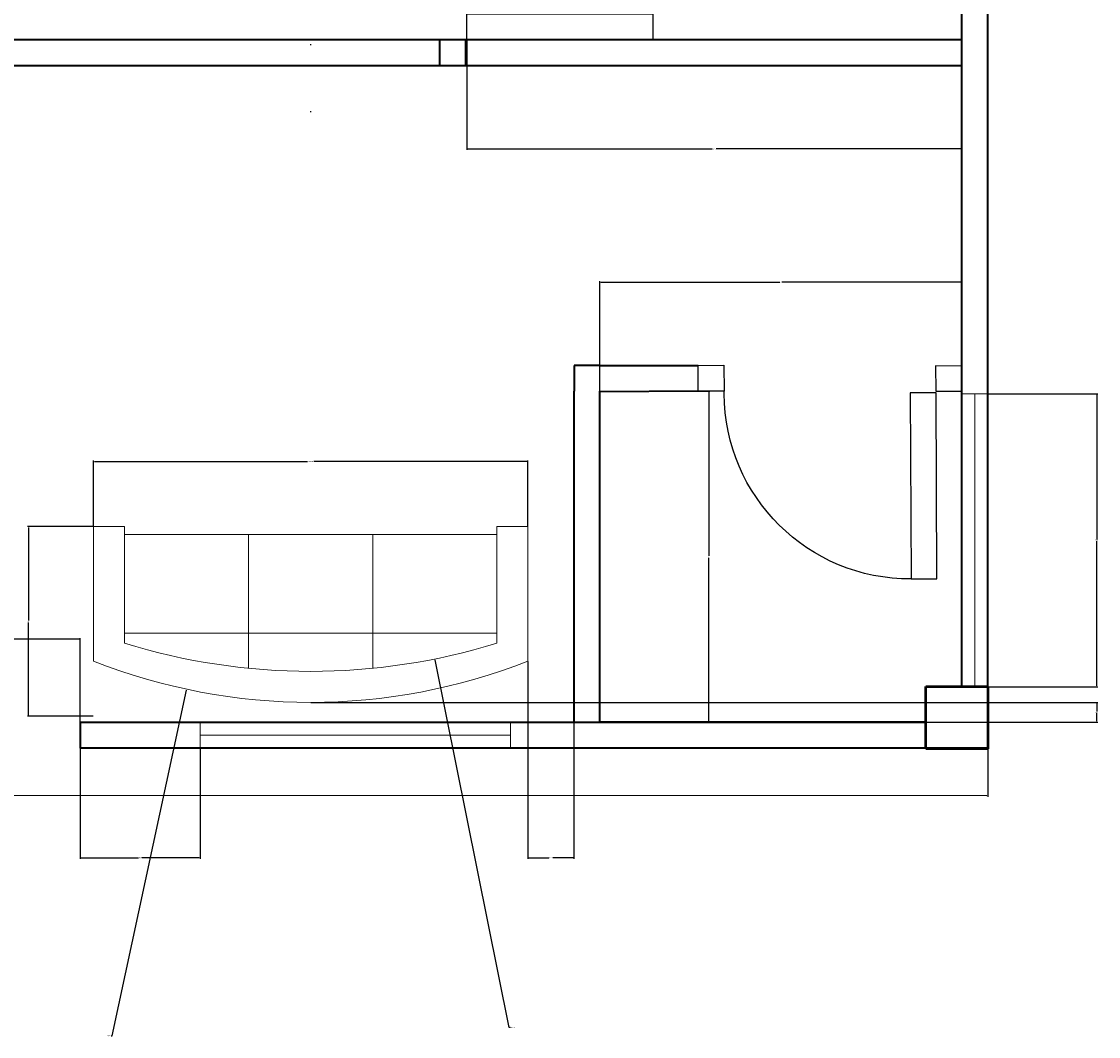
# Model space of a CAD drawing. Units: inches. Extents: x 2082 to 2506, y 790 to 1201.
# Tile 2 of 3: x 2298 to 2506, y 790 to 986. Entities that reach past the tile are written whole.
import ezdxf

# ---------------------------------------------------------------- set-up
doc = ezdxf.new("R2010")
doc.units = ezdxf.units.IN
for name, color, linetype, lineweight in [('A-ANNO-DIMS', 2, 'Continuous', 18), ('A-COLS', 7, 'Continuous', 50), ('A-DOOR', 3, 'Continuous', 25), ('A-FURN', 8, 'Continuous', 18), ('A-GLAZ', 4, 'Continuous', 18), ('A-WALL', 7, 'Continuous', 35)]:
    doc.layers.add(name, color=color, linetype=linetype, lineweight=lineweight)
doc.styles.get("Standard").update_dxf_attribs({"font": 'arial.ttf'})
doc.dimstyles.get("Standard").update_dxf_attribs({"dimtxt": 0.18, "dimasz": 0.18, "dimexe": 0.18, "dimexo": 0.0625, "dimgap": 0.09, "dimtad": 0, "dimtih": 1, "dimtoh": 1, "dimdec": 4, "dimzin": 0, "dimdsep": 46, "dimlunit": 4, "dimtxsty": 'Standard', "dimcen": 0.09, "dimadec": 0, "dimazin": 0, "dimtfac": 1, "dimtdec": 4, "dimtofl": 0, "dimtmove": 0, "dimatfit": 3, "dimfxl": 1, "dimtolj": 1, "dimtzin": 0, "dimarcsym": 0})

# ---------------------------------------------------------------- blocks, each defined once
blk = doc.blocks.new('Sofa - Roundback 7 ft.')
for p, q in [((-12.00002, -32.4421), (-12.00003, -6.5971)), ((11.99997, -32.4421), (11.99998, -6.5971)), ((-36.000027, -34), (-36.000027, -11.4696)), ((35.99998, -34), (35.99998, -11.4696)), ((-35.999844, -13.3819), (35.9998, -13.3819)), ((-36.000027, -32.4421), (35.99998, -32.4421))]:
    blk.add_line(p, q)
for points in [[(-36.000027, -34), (-42.000027, -34), (-42.000027, -8)], [(41.99998, -8), (41.99998, -34), (35.99998, -34)]]:
    blk.add_lwpolyline(points)
for centre, radius, start, end in [((0, -114.25), 114.25, 68.43141, 111.5686), ((-0.00001, -127.1968), 121.1968, 72.72033, 107.2797)]:
    blk.add_arc(centre, radius, start, end)
blk = doc.blocks.new('DOOR-SWING-36IN')
for p, q in [((0, 0), (0, 5)), ((0, 5), (36, 5)), ((36, 5), (36, 0)), ((36, 0), (0, 0))]:
    blk.add_line(p, q)
blk.add_arc((0, 5), 36, 0, 90)
blk = doc.blocks.new('WIN-60IN')
for p, q in [((0, 5), (12, 5)), ((0, 5), (0, 0)), ((12, 5), (60, 5)), ((60, 5), (60, 0)), ((0, 2.5), (60, 2.5)), ((0, 0), (60, 0))]:
    blk.add_line(p, q)
blk = doc.blocks.new('COL-12X12IN')
for p, q in [((0, 12), (12, 12)), ((0, 0), (0, 12)), ((12, 12), (12, 0)), ((12, 0), (0, 0))]:
    blk.add_line(p, q)
blk = doc.blocks.new('*D22')
at = {"layer": 'A-ANNO-DIMS', "color": 0, "lineweight": -2, "transparency": 16777216}
for p, q in [((2311.99, 888.4), (2311.99, 901.12)), ((2312.17, 900.94), (2353.4, 900.94)), ((2395.81, 900.94), (2354.59, 900.94)), ((2395.99, 888.4), (2395.99, 901.12))]:
    blk.add_line(p, q, dxfattribs=at)
at = {"layer": 'A-ANNO-DIMS', "color": 0, "transparency": 16777216}
for points in [[(2312.17, 900.97), (2312.17, 900.91), (2311.99, 900.94)], [(2395.81, 900.97), (2395.81, 900.91), (2395.99, 900.94)]]:
    blk.add_solid(points, dxfattribs=at)
at = {"layer": 'Defpoints', "color": 0, "transparency": 16777216}
for p in [(2311.99, 900.94), (2311.99, 888.34), (2395.99, 888.34)]:
    blk.add_point(p, dxfattribs=at)
at = {"layer": 'A-ANNO-DIMS', "color": 0, "transparency": 16777216, "insert": (2353.99, 900.94), "char_height": 0.18, "attachment_point": 5}
blk.add_mtext('\\A1;SOFA 84', dxfattribs=at)
blk = doc.blocks.new('*D23')
at = {"layer": 'A-ANNO-DIMS', "color": 0, "lineweight": -2, "transparency": 16777216}
for p, q in [((2311.93, 888.34), (2299.21, 888.34)), ((2299.39, 888.16), (2299.39, 870.19)), ((2299.39, 851.85), (2299.39, 869.82)), ((2311.93, 851.67), (2299.21, 851.67))]:
    blk.add_line(p, q, dxfattribs=at)
at = {"layer": 'A-ANNO-DIMS', "color": 0, "transparency": 16777216}
for points in [[(2299.36, 888.16), (2299.42, 888.16), (2299.39, 888.34)], [(2299.36, 851.85), (2299.42, 851.85), (2299.39, 851.67)]]:
    blk.add_solid(points, dxfattribs=at)
at = {"layer": 'Defpoints', "color": 0, "transparency": 16777216}
for p in [(2311.99, 888.34), (2299.39, 851.67), (2311.99, 851.67)]:
    blk.add_point(p, dxfattribs=at)
at = {"layer": 'A-ANNO-DIMS', "color": 0, "transparency": 16777216, "insert": (2299.39, 870), "char_height": 0.18, "attachment_point": 5}
blk.add_mtext('\\A1;37', dxfattribs=at)
blk = doc.blocks.new('*D24')
at = {"layer": 'A-ANNO-DIMS', "color": 0, "lineweight": -2, "transparency": 16777216}
for p, q in [((2102.92, 857.43), (2102.92, 836.21)), ((2484.95, 857.32), (2484.95, 836.1)), ((2103.1, 836.39), (2293.64, 836.34)), ((2484.77, 836.28), (2294.22, 836.34))]:
    blk.add_line(p, q, dxfattribs=at)
at = {"layer": 'A-ANNO-DIMS', "color": 0, "transparency": 16777216}
for points in [[(2103.1, 836.42), (2103.1, 836.36), (2102.92, 836.39)], [(2484.77, 836.31), (2484.77, 836.25), (2484.95, 836.28)]]:
    blk.add_solid(points, dxfattribs=at)
at = {"layer": 'Defpoints', "color": 0, "transparency": 16777216}
for p in [(2102.92, 857.49), (2484.95, 857.38), (2102.92, 836.39)]:
    blk.add_point(p, dxfattribs=at)
at = {"layer": 'A-ANNO-DIMS', "color": 0, "transparency": 16777216, "insert": (2293.93, 836.34), "char_height": 0.18, "attachment_point": 5}
blk.add_mtext('\\A1;382', dxfattribs=at)
blk = doc.blocks.new('*D36')
at = {"layer": 'A-ANNO-DIMS', "color": 0, "lineweight": -2, "transparency": 16777216}
for p, q in [((2384.17, 982.44), (2384.17, 961.22)), ((2479.92, 982.44), (2479.92, 961.22)), ((2384.35, 961.4), (2431.65, 961.4)), ((2479.74, 961.4), (2432.44, 961.4))]:
    blk.add_line(p, q, dxfattribs=at)
at = {"layer": 'A-ANNO-DIMS', "color": 0, "transparency": 16777216}
for points in [[(2384.35, 961.43), (2384.35, 961.37), (2384.17, 961.4)], [(2479.74, 961.43), (2479.74, 961.37), (2479.92, 961.4)]]:
    blk.add_solid(points, dxfattribs=at)
at = {"layer": 'Defpoints', "color": 0, "transparency": 16777216}
for p in [(2384.17, 982.5), (2479.92, 982.5), (2384.17, 961.4)]:
    blk.add_point(p, dxfattribs=at)
at = {"layer": 'A-ANNO-DIMS', "color": 0, "transparency": 16777216, "insert": (2432.05, 961.4), "char_height": 0.18, "attachment_point": 5}
blk.add_mtext('\\A1;95.75', dxfattribs=at)
blk = doc.blocks.new('*D37')
at = {"layer": 'A-ANNO-DIMS', "color": 0, "lineweight": -2, "transparency": 16777216}
for p, q in [((2409.92, 914.56), (2409.92, 935.78)), ((2410.1, 935.6), (2444.71, 935.6)), ((2479.74, 935.6), (2445.14, 935.6)), ((2479.92, 914.56), (2479.92, 935.78))]:
    blk.add_line(p, q, dxfattribs=at)
at = {"layer": 'A-ANNO-DIMS', "color": 0, "transparency": 16777216}
for points in [[(2410.1, 935.63), (2410.1, 935.57), (2409.92, 935.6)], [(2479.74, 935.63), (2479.74, 935.57), (2479.92, 935.6)]]:
    blk.add_solid(points, dxfattribs=at)
at = {"layer": 'Defpoints', "color": 0, "transparency": 16777216}
for p in [(2479.92, 935.6), (2409.92, 914.5), (2479.92, 914.5)]:
    blk.add_point(p, dxfattribs=at)
at = {"layer": 'A-ANNO-DIMS', "color": 0, "transparency": 16777216, "insert": (2444.92, 935.6), "char_height": 0.18, "attachment_point": 5}
blk.add_mtext('\\A1;70', dxfattribs=at)
blk = doc.blocks.new('*D38')
at = {"layer": 'A-ANNO-DIMS', "color": 0, "lineweight": -2, "transparency": 16777216}
for p, q in [((2409.99, 914.5), (2431.2, 914.5)), ((2431.02, 914.32), (2431.02, 882.68)), ((2431.02, 850.68), (2431.02, 882.32)), ((2409.99, 850.5), (2431.2, 850.5))]:
    blk.add_line(p, q, dxfattribs=at)
at = {"layer": 'A-ANNO-DIMS', "color": 0, "transparency": 16777216}
for points in [[(2430.99, 914.32), (2431.05, 914.32), (2431.02, 914.5)], [(2430.99, 850.68), (2431.05, 850.68), (2431.02, 850.5)]]:
    blk.add_solid(points, dxfattribs=at)
at = {"layer": 'Defpoints', "color": 0, "transparency": 16777216}
for p in [(2409.92, 914.5), (2409.92, 850.5), (2431.02, 850.5)]:
    blk.add_point(p, dxfattribs=at)
at = {"layer": 'A-ANNO-DIMS', "color": 0, "transparency": 16777216, "insert": (2431.02, 882.5), "char_height": 0.18, "attachment_point": 5}
blk.add_mtext('\\A1;64', dxfattribs=at)
blk = doc.blocks.new('*D41')
at = {"layer": 'A-ANNO-DIMS', "color": 0, "lineweight": -2, "transparency": 16777216}
for p, q in [((2243.9, 845.56), (2243.9, 866.78)), ((2244.08, 866.6), (2276.28, 866.6)), ((2309.24, 866.6), (2277.04, 866.6)), ((2309.42, 845.56), (2309.42, 866.78))]:
    blk.add_line(p, q, dxfattribs=at)
at = {"layer": 'A-ANNO-DIMS', "color": 0, "transparency": 16777216}
for points in [[(2244.08, 866.63), (2244.08, 866.57), (2243.9, 866.6)], [(2309.24, 866.63), (2309.24, 866.57), (2309.42, 866.6)]]:
    blk.add_solid(points, dxfattribs=at)
at = {"layer": 'Defpoints', "color": 0, "transparency": 16777216}
for p in [(2309.42, 866.6), (2243.9, 845.5), (2309.42, 845.5)]:
    blk.add_point(p, dxfattribs=at)
at = {"layer": 'A-ANNO-DIMS', "color": 0, "transparency": 16777216, "insert": (2276.66, 866.6), "char_height": 0.18, "attachment_point": 5}
blk.add_mtext('\\A1;65.51', dxfattribs=at)
blk = doc.blocks.new('*D43')
at = {"layer": 'A-ANNO-DIMS', "color": 0, "lineweight": -2, "transparency": 16777216}
for p, q in [((2309.42, 845.44), (2309.42, 824.1)), ((2332.62, 845.44), (2332.62, 824.1)), ((2309.6, 824.28), (2320.69, 824.28)), ((2332.44, 824.28), (2321.34, 824.28))]:
    blk.add_line(p, q, dxfattribs=at)
at = {"layer": 'A-ANNO-DIMS', "color": 0, "transparency": 16777216}
for points in [[(2309.6, 824.31), (2309.6, 824.25), (2309.42, 824.28)], [(2332.44, 824.31), (2332.44, 824.25), (2332.62, 824.28)]]:
    blk.add_solid(points, dxfattribs=at)
at = {"layer": 'Defpoints', "color": 0, "transparency": 16777216}
for p in [(2309.42, 845.5), (2332.62, 845.5), (2332.62, 824.28)]:
    blk.add_point(p, dxfattribs=at)
at = {"layer": 'A-ANNO-DIMS', "color": 0, "transparency": 16777216, "insert": (2321.02, 824.28), "char_height": 0.18, "attachment_point": 5}
blk.add_mtext('\\A1;23.2', dxfattribs=at)
blk = doc.blocks.new('*D47')
at = {"layer": 'A-ANNO-DIMS', "color": 0, "lineweight": -2, "transparency": 16777216}
for p, q in [((2484.99, 914), (2506.23, 914)), ((2506.05, 913.82), (2506.05, 885.87)), ((2506.05, 857.56), (2506.05, 885.51)), ((2485.02, 857.38), (2506.23, 857.38))]:
    blk.add_line(p, q, dxfattribs=at)
at = {"layer": 'A-ANNO-DIMS', "color": 0, "transparency": 16777216}
for points in [[(2506.02, 913.82), (2506.08, 913.82), (2506.05, 914)], [(2506.02, 857.56), (2506.08, 857.56), (2506.05, 857.38)]]:
    blk.add_solid(points, dxfattribs=at)
at = {"layer": 'Defpoints', "color": 0, "transparency": 16777216}
for p in [(2484.92, 914), (2506.05, 914), (2484.95, 857.38)]:
    blk.add_point(p, dxfattribs=at)
at = {"layer": 'A-ANNO-DIMS', "color": 0, "transparency": 16777216, "insert": (2506.05, 885.69), "char_height": 0.18, "attachment_point": 5}
blk.add_mtext('\\A1;56.62', dxfattribs=at)
blk = doc.blocks.new('*D54')
at = {"layer": 'A-ANNO-DIMS', "color": 0, "lineweight": -2, "transparency": 16777216}
for p, q in [((2395.99, 862.27), (2395.99, 824.1)), ((2404.92, 850.44), (2404.92, 824.1)), ((2396.17, 824.28), (2400.06, 824.28)), ((2404.74, 824.28), (2400.85, 824.28))]:
    blk.add_line(p, q, dxfattribs=at)
at = {"layer": 'A-ANNO-DIMS', "color": 0, "transparency": 16777216}
for points in [[(2396.17, 824.31), (2396.17, 824.25), (2395.99, 824.28)], [(2404.74, 824.31), (2404.74, 824.25), (2404.92, 824.28)]]:
    blk.add_solid(points, dxfattribs=at)
at = {"layer": 'Defpoints', "color": 0, "transparency": 16777216}
for p in [(2395.99, 862.34), (2404.92, 850.5), (2404.92, 824.28)]:
    blk.add_point(p, dxfattribs=at)
at = {"layer": 'A-ANNO-DIMS', "color": 0, "transparency": 16777216, "insert": (2400.46, 824.28), "char_height": 0.18, "attachment_point": 5}
blk.add_mtext('\\A1;8.933', dxfattribs=at)
blk = doc.blocks.new('*D55')
at = {"layer": 'A-ANNO-DIMS', "color": 0, "lineweight": -2, "transparency": 16777216}
for p, q in [((2354.05, 854.34), (2506.23, 854.34)), ((2506.05, 854.16), (2506.05, 852.6)), ((2506.05, 850.68), (2506.05, 852.24)), ((2404.99, 850.5), (2506.23, 850.5))]:
    blk.add_line(p, q, dxfattribs=at)
at = {"layer": 'A-ANNO-DIMS', "color": 0, "transparency": 16777216}
for points in [[(2506.02, 854.16), (2506.08, 854.16), (2506.05, 854.34)], [(2506.02, 850.68), (2506.08, 850.68), (2506.05, 850.5)]]:
    blk.add_solid(points, dxfattribs=at)
at = {"layer": 'Defpoints', "color": 0, "transparency": 16777216}
for p in [(2353.99, 854.34), (2404.92, 850.5), (2506.05, 850.5)]:
    blk.add_point(p, dxfattribs=at)
at = {"layer": 'A-ANNO-DIMS', "color": 0, "transparency": 16777216, "insert": (2506.05, 852.42), "char_height": 0.18, "attachment_point": 5}
blk.add_mtext('\\A1;3.838', dxfattribs=at)
blk = doc.blocks.new('*D58')
at = {"layer": 'A-ANNO-DIMS', "color": 0, "lineweight": -2, "transparency": 16777216}
for p, q in [((2353.9, 981.53), (2354.08, 981.53)), ((2353.99, 981.44), (2353.99, 981.62)), ((2392.41, 791.46), (2378.04, 862.56)), ((2392.59, 791.46), (2392.41, 791.46))]:
    blk.add_line(p, q, dxfattribs=at)
at = {"layer": 'A-ANNO-DIMS', "color": 0, "transparency": 16777216}
blk.add_solid([(2378.07, 862.57), (2378.01, 862.56), (2378, 862.74)], dxfattribs=at)
at = {"layer": 'Defpoints', "color": 0, "transparency": 16777216}
for p in [(2353.99, 981.53), (2378, 862.74)]:
    blk.add_point(p, dxfattribs=at)
at = {"layer": 'A-ANNO-DIMS', "color": 0, "transparency": 16777216, "insert": (2393.06, 791.46), "char_height": 0.18, "attachment_point": 5}
blk.add_mtext('\\A1;R121.2', dxfattribs=at)
blk = doc.blocks.new('*D59')
at = {"layer": 'A-ANNO-DIMS', "color": 0, "lineweight": -2, "transparency": 16777216}
for p, q in [((2353.9, 968.59), (2354.08, 968.59)), ((2353.99, 968.5), (2353.99, 968.68)), ((2315.61, 789.86), (2329.96, 856.71)), ((2315.43, 789.86), (2315.61, 789.86))]:
    blk.add_line(p, q, dxfattribs=at)
at = {"layer": 'A-ANNO-DIMS', "color": 0, "transparency": 16777216}
blk.add_solid([(2329.93, 856.71), (2329.99, 856.7), (2330, 856.88)], dxfattribs=at)
at = {"layer": 'Defpoints', "color": 0, "transparency": 16777216}
for p in [(2353.99, 968.59), (2330, 856.88)]:
    blk.add_point(p, dxfattribs=at)
at = {"layer": 'A-ANNO-DIMS', "color": 0, "transparency": 16777216, "insert": (2314.88, 789.86), "char_height": 0.18, "attachment_point": 5}
blk.add_mtext('\\A1;R114.25', dxfattribs=at)

msp = doc.modelspace()

# ---------------------------------------------------------------- linework, layer by layer
at = {"layer": 'A-DOOR'}
for p, q in [((2378.9236, 982.4988), (2378.9236, 977.4988)), ((2383.9236, 982.4988), (2378.9236, 982.4988)), ((2378.9236, 982.4988), (2378.9236, 977.4988)), ((2383.9236, 977.4988), (2383.9236, 982.4988)), ((2383.9236, 982.4988), (2383.9236, 977.4988)), ((2378.9236, 977.4988), (2383.9236, 977.4988)), ((2428.923, 919.4988), (2433.923, 919.523)), ((2428.9473, 914.4988), (2428.923, 919.4988)), ((2433.923, 919.523), (2433.9472, 914.523)), ((2474.9479, 914.4747), (2474.9237, 919.4746)), ((2474.9238, 919.4504), (2479.9236, 919.4988)), ((2479.9236, 919.4988), (2479.9478, 914.4989)), ((2479.9236, 919.4988), (2479.9478, 914.4989)), ((2433.9472, 914.523), (2428.9473, 914.4988)), ((2433.9496, 914.0293), (2433.9472, 914.523)), ((2474.9478, 914.4988), (2479.9236, 914.4988)), ((2479.9478, 914.4989), (2474.9479, 914.4747))]:
    msp.add_line(p, q, dxfattribs=at)
at = {"layer": 'A-GLAZ'}
for p, q in [((2484.9236, 913.9988), (2479.9236, 913.9988)), ((2479.9236, 913.9988), (2479.9236, 857.3835)), ((2482.4236, 913.9988), (2482.4236, 857.3835)), ((2484.9236, 913.9988), (2484.9236, 901.9988)), ((2484.9236, 901.9988), (2484.9236, 853.9988))]:
    msp.add_line(p, q, dxfattribs=at)
at = {"layer": 'A-WALL'}
for p, q in [((2484.9236, 1179.4988), (2484.9236, 850.4988)), ((2479.9236, 977.4988), (2479.9236, 1049.4988)), ((2243.9236, 982.4988), (2479.9236, 982.4988)), ((2378.9236, 982.4988), (2378.9236, 977.4988)), ((2243.9236, 977.4988), (2479.9236, 977.4988)), ((2479.9236, 857.3835), (2479.9236, 977.4988)), ((2409.9236, 919.4988), (2404.9236, 919.4988)), ((2404.9236, 919.4988), (2404.9236, 914.4988)), ((2409.9236, 919.4988), (2428.923, 919.4988)), ((2404.9236, 850.4988), (2404.9236, 914.4988)), ((2409.9236, 850.4988), (2409.9236, 914.4988)), ((2428.9473, 914.4988), (2409.9236, 914.4067)), ((2309.4173, 850.4988), (2409.9236, 850.4988)), ((2309.4173, 850.4988), (2309.4173, 845.4988)), ((2409.9236, 850.4988), (2472.9535, 850.4988)), ((2472.9535, 850.4988), (2409.9236, 850.4988)), ((2484.9236, 850.4988), (2484.9236, 845.4988)), ((2484.9236, 845.4988), (2309.4173, 845.4988))]:
    msp.add_line(p, q, dxfattribs=at)

# ---------------------------------------------------------------- block references
at = {"layer": 'A-COLS', "rotation": 90.00000000000216}
msp.add_blockref('COL-12X12IN', (2484.9535, 845.3835), dxfattribs=at)
at = {"layer": 'A-DOOR'}
msp.add_blockref('DOOR-SWING-36IN', (2384.1705, 982.4988), dxfattribs=at)
at = {"layer": 'A-DOOR', "extrusion": (0, 0, -1), "zscale": -1, "rotation": 269.722629678645}
msp.add_blockref('DOOR-SWING-36IN', (-2474.9491, 914.2278), dxfattribs=at)
at = {"layer": 'A-FURN', "rotation": 180}
msp.add_blockref('Sofa - Roundback 7 ft.', (2353.9908, 854.3371), dxfattribs=at)
at = {"layer": 'A-GLAZ'}
msp.add_blockref('WIN-60IN', (2332.6188, 845.4988), dxfattribs=at)

# ---------------------------------------------------------------- dimensions: what is measured, and where the dimension line sits
at = {"layer": 'A-ANNO-DIMS'}
for center, mpoint, override, picture, middle in [((2353.9908, 981.5339), (2378.0002, 862.739), {"dimdec": 1, "dimlfac": 1, "dimrnd": 0, "dimzin": 0, "dimdsep": 46, "dimlunit": 2}, '*D58', (2393.0647, 791.4621)), ((2353.9908, 968.5871), (2330.0009, 856.8841), {"dimdec": 2, "dimlfac": 1, "dimrnd": 0, "dimzin": 0, "dimdsep": 46, "dimlunit": 2}, '*D59', (2314.8765, 789.8624))]:
    dim = msp.add_radius_dim(center=center, mpoint=mpoint, dimstyle='Standard', override=override, dxfattribs=at)
    dim.commit()
    dim.dimension.update_dxf_attribs({"geometry": picture, "text_midpoint": middle, "dimtype": 164})
for base, p1, p2, angle, override, picture, middle in [((2384.1705, 961.3988), (2479.9236, 982.4988), (2384.1705, 982.4988), 180, {"dimdec": 2, "dimlfac": 1, "dimrnd": 0, "dimzin": 0, "dimdsep": 46, "dimlunit": 2}, '*D36', (2432.0471, 961.3988)), ((2431.0236, 850.4988), (2409.9236, 914.4988), (2409.9236, 850.4988), 270, {"dimdec": 0, "dimlfac": 1, "dimrnd": 0, "dimzin": 0, "dimdsep": 46, "dimlunit": 2}, '*D38', (2431.0236, 882.4988)), ((2506.0535, 913.9988), (2484.9535, 857.3835), (2484.9236, 913.9988), 90, {"dimdec": 2, "dimlfac": 1, "dimrnd": 0, "dimzin": 0, "dimdsep": 46, "dimlunit": 2}, '*D47', (2506.0535, 885.6911)), ((2299.3908, 851.6704), (2311.9908, 888.3371), (2311.9908, 851.6704), 270, {"dimdec": 0, "dimlfac": 1, "dimrnd": 0, "dimzin": 0, "dimdsep": 46, "dimlunit": 2}, '*D23', (2299.3908, 870.0037)), ((2102.9176, 836.3921), (2484.9535, 857.3835), (2102.9236, 857.4921), 179.98371, {"dimdec": 0, "dimlfac": 1, "dimrnd": 0, "dimzin": 0, "dimdsep": 46, "dimlunit": 2}, '*D24', (2293.9326, 836.3378)), ((2506.0535, 850.4988), (2353.9908, 854.3371), (2404.9236, 850.4988), 90, {"dimdec": 3, "dimlfac": 1, "dimrnd": 0, "dimzin": 0, "dimdsep": 46, "dimlunit": 2}, '*D55', (2506.0535, 852.4179))]:
    dim = msp.add_linear_dim(base=base, p1=p1, p2=p2, angle=angle, dimstyle='Standard', override=override, dxfattribs=at)
    dim.commit()
    dim.dimension.update_dxf_attribs({"geometry": picture, "text_midpoint": middle})
for base, p1, p2, override, picture, middle in [((2479.9236, 935.5988), (2409.9236, 914.4988), (2479.9236, 914.4988), {"dimdec": 0, "dimlfac": 1, "dimrnd": 0, "dimzin": 0, "dimdsep": 46, "dimlunit": 2}, '*D37', (2444.9236, 935.5988)), ((2309.4173, 866.5988), (2243.9029, 845.4988), (2309.4173, 845.4988), {"dimdec": 2, "dimlfac": 1, "dimrnd": 0, "dimzin": 0, "dimdsep": 46, "dimlunit": 2}, '*D41', (2276.6601, 866.5988)), ((2404.9236, 824.2835), (2395.9908, 862.3371), (2404.9236, 850.4988), {"dimdec": 3, "dimlfac": 1, "dimrnd": 0, "dimzin": 0, "dimdsep": 46, "dimlunit": 2}, '*D54', (2400.4572, 824.2835)), ((2332.6188, 824.2835), (2309.4173, 845.4988), (2332.6188, 845.4988), {"dimdec": 1, "dimlfac": 1, "dimrnd": 0, "dimzin": 0, "dimdsep": 46, "dimlunit": 2}, '*D43', (2321.0181, 824.2835))]:
    dim = msp.add_linear_dim(base=base, p1=p1, p2=p2, dimstyle='Standard', override=override, dxfattribs=at)
    dim.commit()
    dim.dimension.update_dxf_attribs({"geometry": picture, "text_midpoint": middle})
dim = msp.add_linear_dim(base=(2311.9908, 900.9371), p1=(2395.9908, 888.3371), p2=(2311.9908, 888.3371), angle=180, text='SOFA <>', dimstyle='Standard', override={"dimdec": 0, "dimlfac": 1, "dimrnd": 0, "dimzin": 0, "dimdsep": 46, "dimlunit": 2}, dxfattribs=at)
dim.commit()
dim.dimension.update_dxf_attribs({"geometry": '*D22', "text_midpoint": (2353.9908, 900.9371)})

doc.saveas('drawing.dxf')
